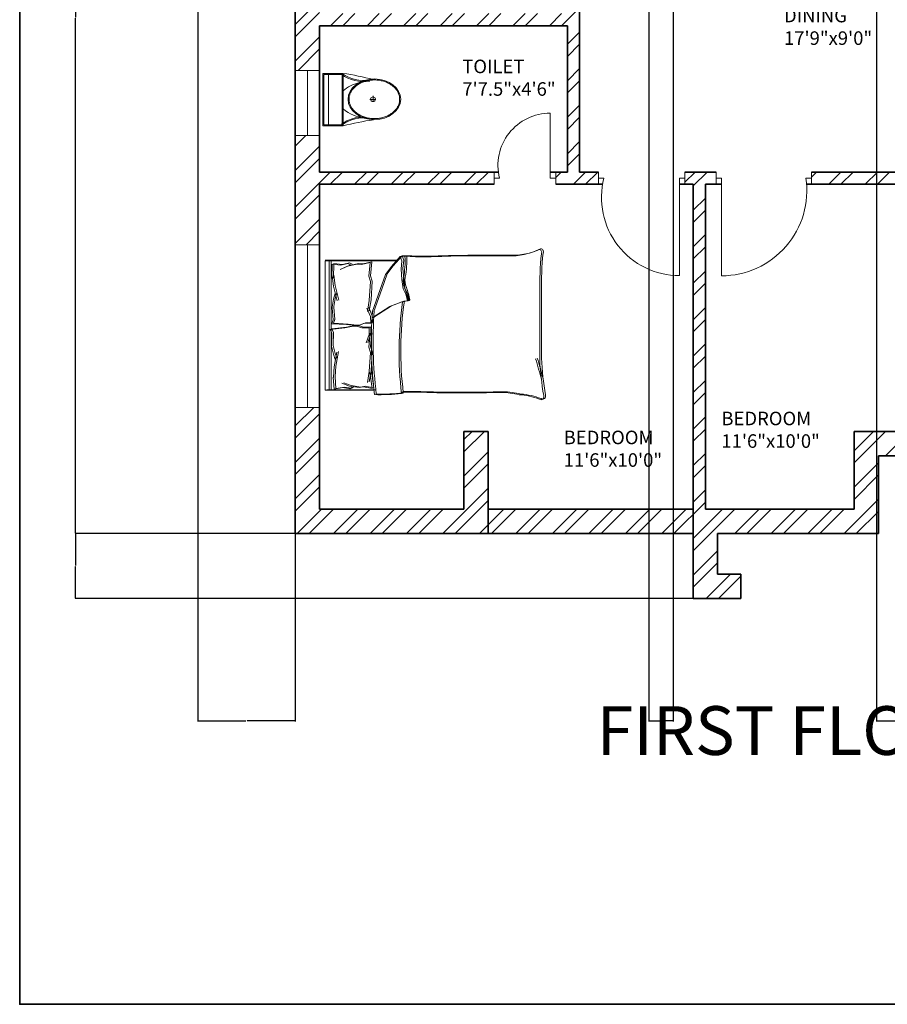
# Model space of a CAD drawing. Units: inches. Extents: x 1513 to 2170, y 1240 to 2288.
# Tile 1 of 10: x 1513 to 1834, y 1240 to 1603. Entities that reach past the tile are written whole.
import ezdxf

# ---------------------------------------------------------------- set-up
doc = ezdxf.new("R2010")
doc.units = ezdxf.units.IN
for name, color, linetype, lineweight in [('A-ANNO-DIMS', 2, 'Continuous', 18), ('A-ANNO-TTLB', 7, 'Continuous', 35), ('A-AREA-IDEN', 7, 'Continuous', 18), ('A-DOOR', 3, 'Continuous', 18), ('A-FLOR-FIXT', 9, 'Continuous', 18), ('A-FURN', 8, 'Continuous', 18), ('A-GLAZ', 4, 'Continuous', 18), ('A-WALL', 7, 'Continuous', 35), ('A-WALL-PATT', 252, 'Continuous', 13)]:
    doc.layers.add(name, color=color, linetype=linetype, lineweight=lineweight)
doc.styles.get("Standard").update_dxf_attribs({"font": 'arial.ttf'})
doc.dimstyles.get("Standard").update_dxf_attribs({"dimtxt": 0.18, "dimasz": 0.18, "dimexe": 0.18, "dimexo": 0.0625, "dimgap": 0.09, "dimtad": 0, "dimtih": 1, "dimtoh": 1, "dimdec": 4, "dimzin": 0, "dimdsep": 46, "dimtxsty": 'Standard', "dimcen": 0.09, "dimadec": 0, "dimazin": 0, "dimtfac": 1, "dimtdec": 4, "dimtofl": 0, "dimtmove": 0, "dimatfit": 3, "dimfxl": 1, "dimtolj": 1, "dimtzin": 0, "dimarcsym": 0})

# ---------------------------------------------------------------- blocks, each defined once
blk = doc.blocks.new('A$C31115884')
for p, q in [((283.1, 497.7), (223.4, 497.7)), ((257.5, 466.4), (257.5, 523.2)), ((0, 200), (0, 0)), ((520, 200), (0, 200)), ((520, 0), (520, 200)), ((10, 190), (10, 10)), ((510, 190), (10, 190)), ((510, 10), (510, 190)), ((510, 54.5), (0, 54.5)), ((10, 10), (510, 10)), ((0, 0), (520, 0))]:
    blk.add_line(p, q)
blk.add_circle((255.6, 496.4), 23.6)
for centre, radius, start, end in [((2777.7, -204.6), 2807, 165.4549, 171.71327), ((3237, 905), 2807, 188.28673, 194.5451), ((-294.5, 403.3), 364.7, 324.20913, 9.34987), ((-294.5, 403.3), 374.7, 324.20913, 9.34987), ((139.5, 406.2), 293.5, 315.84364, 2.65635), ((805.8, 403.3), 374.7, 179.20365, 215.79087), ((805.8, 403.3), 364.7, 170.65013, 215.79087), ((383.6, 406.2), 293.5, 190.27735, 224.15636)]:
    blk.add_arc(centre, radius, start, end)
blk.add_ellipse((256.2, 509.9), major_axis=(0, -260.7), ratio=0.772727)
blk.add_open_spline([(256.2, 259.2), (263.1, 259.2), (270, 259.7), (287.8, 262.3), (298.7, 265.1), (319.9, 273.1), (330.2, 278.4), (350.1, 291.1), (359.7, 298.7), (377.7, 315.9), (386.2, 325.5), (401.7, 346.6), (408.8, 358.1), (421.3, 382.5), (426.8, 395.5), (435.9, 422.4), (439.5, 436.4), (444.8, 465.1), (446.5, 479.7), (447.9, 509.2), (447.6, 524), (445, 553.3), (442.7, 567.8), (436.3, 596), (432.1, 609.7), (421.9, 636), (416, 648.6), (402.5, 672.1), (395, 683), (378.6, 703), (369.8, 712.1), (351.1, 728), (341.3, 734.8), (320.9, 746.2), (310.4, 750.7), (288.9, 757.3), (278, 759.4), (256, 761), (245, 760.6), (223.1, 757.2), (212.3, 754.3), (191.1, 746.1), (180.8, 740.7), (160.9, 727.8), (151.4, 720.1), (133.5, 702.7), (125.1, 693), (109.6, 671.7), (102.6, 660.2), (90.2, 635.7), (84.9, 622.7), (76, 595.6), (72.4, 581.6), (67.2, 552.9), (65.6, 538.2), (64.4, 508.8), (64.8, 494), (67.5, 464.7), (69.9, 450.2), (76.6, 422), (80.8, 408.3), (91.1, 382.2), (97.2, 369.7), (110.8, 346.3), (118.4, 335.4), (134.8, 315.6), (143.7, 306.7), (162.4, 290.9), (172.3, 284.2), (192.8, 273), (203.3, 268.6), (224.8, 262.2), (235.8, 260.2), (249.9, 259.3), (253, 259.2), (256.2, 259.2)], degree=3, knots=[0, 0, 0, 0, 0.110105, 0.110105, 0.285049, 0.285049, 0.459994, 0.459994, 0.634938, 0.634938, 0.809882, 0.809882, 0.984827, 0.984827, 1.159771, 1.159771, 1.334715, 1.334715, 1.50966, 1.50966, 1.684604, 1.684604, 1.859549, 1.859549, 2.034493, 2.034493, 2.209437, 2.209437, 2.384382, 2.384382, 2.559326, 2.559326, 2.73427, 2.73427, 2.909215, 2.909215, 3.084159, 3.084159, 3.259103, 3.259103, 3.434048, 3.434048, 3.608992, 3.608992, 3.783936, 3.783936, 3.958881, 3.958881, 4.133825, 4.133825, 4.30877, 4.30877, 4.483714, 4.483714, 4.658658, 4.658658, 4.833603, 4.833603, 5.008547, 5.008547, 5.183491, 5.183491, 5.358436, 5.358436, 5.53338, 5.53338, 5.708324, 5.708324, 5.883269, 5.883269, 6.058213, 6.058213, 6.233158, 6.233158, 6.283185, 6.283185, 6.283185, 6.283185])
blk = doc.blocks.new('BED-DOUBLE')
for p, q in [((0, 51.27), (26.61, 51.27)), ((0, 51.27), (26.61, 51.27)), ((0.64, 51.49), (27.25, 51.49)), ((0.64, 51.49), (27.25, 51.49)), ((1.53, 3.48), (1.53, 51.27)), ((1.53, 3.48), (1.53, 51.27)), ((2.17, 3.7), (2.17, 51.49)), ((2.17, 3.7), (2.17, 51.49)), ((17.21, 50.93), (14.07, 50.15)), ((17.21, 50.93), (14.07, 50.15)), ((16.8, 45.8), (17.21, 50.93)), ((16.8, 45.8), (17.21, 50.93)), ((27.74, 52.87), (24.49, 49.16)), ((27.74, 52.87), (24.49, 49.16)), ((28.38, 53.1), (25.13, 49.39)), ((28.38, 53.1), (25.13, 49.39)), ((29.49, 52.95), (27.74, 52.87, 3.87)), ((29.49, 52.95), (27.74, 52.87, 3.87)), ((28.36, 51.33), (27.74, 52.87)), ((28.36, 51.33), (27.74, 52.87)), ((28.05, 48.23), (28.36, 51.33)), ((28.05, 48.23), (28.36, 51.33)), ((30.13, 53.18), (28.38, 53.1, 3.87)), ((30.13, 53.18), (28.38, 53.1, 3.87)), ((29, 51.56), (28.38, 53.1)), ((29, 51.56), (28.38, 53.1)), ((28.69, 48.46), (29, 51.56)), ((28.69, 48.46), (29, 51.56)), ((2.55, 50.11), (2.46, 44.71)), ((2.55, 50.11), (2.46, 44.71)), ((2.55, 50.11), (5.76, 49.73)), ((2.55, 50.11), (5.76, 49.73)), ((3.19, 50.34), (3.1, 44.94)), ((3.19, 50.34), (3.1, 44.94)), ((3.19, 50.34), (6.4, 49.96)), ((3.19, 50.34), (6.4, 49.96)), ((8.25, 49.31), (5.57, 48.13)), ((8.25, 49.31), (5.57, 48.13)), ((5.76, 49.73), (8.33, 50.33)), ((5.76, 49.73), (8.33, 50.33)), ((8.89, 49.54), (6.21, 48.36)), ((8.89, 49.54), (6.21, 48.36)), ((6.4, 49.96), (8.97, 50.56)), ((6.4, 49.96), (8.97, 50.56)), ((11.83, 50.11), (8.25, 49.31)), ((11.83, 50.11), (8.25, 49.31)), ((8.33, 50.33), (9.38, 49.82)), ((8.33, 50.33), (9.38, 49.82)), ((12.46, 50.34), (8.89, 49.54)), ((12.46, 50.34), (8.89, 49.54)), ((8.97, 50.56), (10.02, 50.04)), ((8.97, 50.56), (10.02, 50.04)), ((13.43, 49.92), (11.83, 50.11)), ((13.43, 49.92), (11.83, 50.11)), ((14.07, 50.15), (12.46, 50.34)), ((14.07, 50.15), (12.46, 50.34)), ((16.57, 50.7), (13.43, 49.92)), ((16.57, 50.7), (13.43, 49.92)), ((16.17, 45.57), (16.57, 50.7)), ((16.17, 45.57), (16.57, 50.7)), ((24.49, 49.16), (22.33, 46.22)), ((24.49, 49.16), (22.33, 46.22)), ((25.13, 49.39), (22.96, 46.45)), ((25.13, 49.39), (22.96, 46.45)), ((28.36, 44.36), (28.05, 48.23)), ((28.36, 44.36), (28.05, 48.23)), ((29, 44.59), (28.69, 48.46)), ((29, 44.59), (28.69, 48.46)), ((2.46, 44.71), (2.54, 45.71)), ((2.46, 44.71), (2.54, 45.71)), ((2.54, 45.71), (3.07, 41.92)), ((2.54, 45.71), (3.07, 41.92)), ((3.1, 44.94), (3.18, 45.94)), ((3.1, 44.94), (3.18, 45.94)), ((3.18, 45.94), (3.71, 42.14)), ((3.18, 45.94), (3.71, 42.14)), ((16.72, 43.61), (16.17, 45.57)), ((16.72, 43.61), (16.17, 45.57)), ((17.36, 43.84), (16.8, 45.8)), ((17.36, 43.84), (16.8, 45.8)), ((16.93, 36.83), (17.36, 43.84)), ((16.93, 36.83), (17.36, 43.84)), ((22.33, 46.22), (20.31, 40.65)), ((22.33, 46.22), (20.31, 40.65)), ((22.96, 46.45), (20.95, 40.87)), ((22.96, 46.45), (20.95, 40.87)), ((28.83, 40.96), (28.36, 44.36)), ((28.83, 40.95), (28.36, 44.36)), ((29.46, 41.18), (29, 44.59)), ((29.46, 41.18), (29, 44.59)), ((3.07, 41.92), (4.42, 36.5)), ((3.07, 41.92), (4.42, 36.5)), ((3.71, 42.14), (5.06, 36.72)), ((3.71, 42.14), (5.06, 36.72)), ((16.29, 36.6), (16.72, 43.61)), ((16.29, 36.6), (16.72, 43.61)), ((20.31, 40.65), (17.38, 32.31)), ((20.31, 40.65), (17.38, 32.31)), ((20.95, 40.87), (18.02, 32.54)), ((20.95, 40.87), (18.02, 32.54)), ((29.75, 38.94), (28.83, 40.96)), ((29.75, 38.94), (28.83, 40.95)), ((30.39, 39.17), (29.46, 41.18)), ((30.39, 39.17), (29.46, 41.18)), ((3.07, 37.14), (2.53, 34.21)), ((3.07, 37.14), (2.53, 34.21)), ((3.67, 39.2), (3.07, 37.14)), ((3.67, 39.2), (3.07, 37.14)), ((3.71, 37.36), (3.17, 34.43)), ((3.71, 37.36), (3.17, 34.43)), ((4.31, 39.43), (3.71, 37.36)), ((4.31, 39.43), (3.71, 37.36)), ((15.62, 32.57), (16.29, 36.6)), ((15.62, 32.57), (16.29, 36.6)), ((16.26, 32.79), (16.93, 36.83)), ((16.26, 32.79), (16.93, 36.83)), ((24.51, 34.68), (29, 36.38)), ((24.51, 34.68), (29, 36.38)), ((28.36, 36.15), (30.37, 36.46)), ((28.36, 36.15), (30.37, 36.46)), ((29, 36.38), (31.01, 36.69)), ((29, 36.38), (31.01, 36.69)), ((30.37, 36.46), (29.75, 38.94)), ((30.37, 36.46), (29.75, 38.94)), ((31.01, 36.69), (30.39, 39.17)), ((31.01, 36.69), (30.39, 39.17)), ((79.24, 15.06), (79.24, 39.68)), ((79.24, 15.06), (79.24, 39.68)), ((79.88, 15.29), (79.88, 39.91)), ((79.88, 15.29), (79.88, 39.91)), ((2.53, 34.21), (2.55, 33.88)), ((2.53, 34.21), (2.55, 33.88)), ((2.55, 33.88), (2.98, 29.46)), ((2.55, 33.88), (2.98, 29.46)), ((3.17, 34.43), (3.19, 34.11)), ((3.17, 34.43), (3.19, 34.11)), ((3.19, 34.11), (3.61, 29.69)), ((3.19, 34.11), (3.61, 29.68)), ((16.74, 30.75), (15.45, 33.82)), ((16.74, 30.75), (15.45, 33.82)), ((17.38, 30.98), (16.09, 34.05)), ((17.38, 30.98), (16.09, 34.05)), ((17.38, 30.26), (23.87, 34.45)), ((17.38, 30.26), (23.87, 34.45)), ((18.02, 30.49), (24.51, 34.68)), ((18.02, 30.49), (24.51, 34.68)), ((23.87, 34.45), (28.36, 36.15)), ((23.87, 34.45), (28.36, 36.15)), ((2.98, 29.46), (2.49, 27.98)), ((2.98, 29.46), (2.49, 27.98)), ((3.61, 29.69), (3.13, 28.21)), ((3.61, 29.68), (3.13, 28.21)), ((16.89, 28.3), (16.74, 30.75)), ((16.89, 28.3), (16.74, 30.75)), ((17.53, 28.53), (17.38, 30.98)), ((17.53, 28.53), (17.38, 30.98)), ((1.87, 25.98), (7.22, 26.56)), ((1.87, 25.98), (7.22, 26.56)), ((2.44, 24.54), (1.87, 25.98)), ((2.44, 24.54), (1.87, 25.98)), ((2.49, 27.98), (7.86, 27.73)), ((2.49, 27.98), (7.86, 27.73)), ((2.51, 26.21), (7.86, 26.79)), ((2.51, 26.21), (7.86, 26.79)), ((3.08, 24.77), (2.51, 26.21)), ((3.08, 24.77), (2.51, 26.21)), ((3.13, 28.21), (8.5, 27.96)), ((3.13, 28.21), (8.5, 27.96)), ((7.22, 26.56), (10.4, 27.14)), ((7.22, 26.56), (10.4, 27.14)), ((7.86, 27.73), (11.07, 27.36)), ((7.86, 27.73), (11.07, 27.36)), ((7.86, 26.79), (11.04, 27.37)), ((7.86, 26.79), (11.04, 27.37)), ((8.5, 27.96), (11.71, 27.58)), ((8.5, 27.96), (11.71, 27.58)), ((10.4, 27.14), (11.7, 27.14)), ((10.4, 27.14), (11.7, 27.14)), ((11.04, 27.37), (12.34, 27.37)), ((11.04, 27.37), (12.34, 27.37)), ((11.07, 27.36), (12.37, 27.44)), ((11.07, 27.36), (12.37, 27.44)), ((11.7, 27.14), (13.58, 26.56)), ((11.7, 27.14), (13.58, 26.56)), ((11.71, 27.58), (13.01, 27.67)), ((11.71, 27.58), (13.01, 27.67)), ((12.34, 27.37), (14.22, 26.79)), ((12.34, 27.37), (14.22, 26.79)), ((12.37, 27.44), (14.21, 28.13)), ((12.37, 27.44), (14.21, 28.13)), ((13.01, 27.67), (14.85, 28.36)), ((13.01, 27.67), (14.85, 28.36)), ((13.58, 26.56), (16.26, 26.56)), ((13.58, 26.56), (16.26, 26.56)), ((14.21, 28.13), (16.89, 28.3)), ((14.21, 28.13), (16.89, 28.3)), ((14.22, 26.79), (16.9, 26.79)), ((14.22, 26.79), (16.9, 26.79)), ((14.85, 28.36), (17.53, 28.53)), ((14.85, 28.36), (17.53, 28.53)), ((16.26, 26.56), (16.26, 24.1)), ((16.26, 26.56), (16.26, 24.1)), ((16.9, 26.79), (16.9, 24.33)), ((16.9, 26.79), (16.9, 24.33)), ((2.3, 20.09), (2.44, 24.54)), ((2.3, 20.09), (2.44, 24.54)), ((2.94, 20.32), (3.08, 24.77)), ((2.94, 20.32), (3.08, 24.77)), ((16.26, 24.1), (15.17, 20.96)), ((16.26, 24.1), (15.17, 20.96)), ((16.9, 24.33), (15.81, 21.19)), ((16.9, 24.33), (15.81, 21.19)), ((16.17, 19.39), (16.57, 24.52)), ((16.17, 19.38), (16.57, 24.52)), ((16.8, 19.61), (17.21, 24.75)), ((16.8, 19.61), (17.21, 24.74)), ((2.3, 19.77), (2.3, 20.09)), ((2.3, 19.77), (2.3, 20.09)), ((3.02, 16.88), (2.3, 19.77)), ((3.02, 16.88), (2.3, 19.77)), ((2.94, 20), (2.94, 20.32)), ((2.94, 20), (2.94, 20.32)), ((3.66, 17.11), (2.94, 20)), ((3.66, 17.11), (2.94, 20)), ((16.72, 17.42), (16.17, 19.39)), ((16.72, 17.42), (16.17, 19.38)), ((17.36, 17.65), (16.8, 19.61)), ((17.36, 17.65), (16.8, 19.61)), ((3.75, 14.86), (3.02, 16.88)), ((3.75, 14.86), (3.02, 16.88)), ((3.31, 12.11), (4.32, 17.6)), ((3.31, 12.11), (4.32, 17.6)), ((4.39, 15.08), (3.66, 17.11)), ((4.39, 15.08), (3.66, 17.11)), ((3.95, 12.34), (4.96, 17.83)), ((3.95, 12.34), (4.96, 17.83)), ((16.29, 10.41), (16.72, 17.42)), ((16.29, 10.41), (16.72, 17.42)), ((16.93, 10.64), (17.36, 17.65)), ((16.93, 10.64), (17.36, 17.65)), ((3.02, 8.29), (3.31, 12.11)), ((3.02, 8.29), (3.31, 12.11)), ((3.66, 8.51), (3.95, 12.34)), ((3.66, 8.51), (3.95, 12.34)), ((3.01, 8.18), (3.02, 8.29)), ((3.01, 8.18), (3.02, 8.29)), ((3.33, 3.9), (3.01, 8.18)), ((3.33, 3.9), (3.01, 8.18)), ((3.64, 8.41), (3.66, 8.51)), ((3.64, 8.41), (3.66, 8.51)), ((3.97, 4.13), (3.64, 8.41)), ((3.97, 4.13), (3.64, 8.41)), ((15.62, 6.38), (16.29, 10.41)), ((15.62, 6.38), (16.29, 10.41)), ((16.26, 6.61), (16.93, 10.64)), ((16.26, 6.61), (16.93, 10.64)), ((16.29, 10.41), (16.61, 9.28)), ((16.29, 10.41), (16.61, 9.28)), ((16.61, 9.28), (17.34, 4.18)), ((16.61, 9.28), (17.34, 4.18)), ((16.93, 10.64), (17.25, 9.51)), ((16.93, 10.64), (17.25, 9.51)), ((17.25, 9.51), (17.98, 4.41)), ((17.25, 9.51), (17.98, 4.41)), ((18.75, 3.7), (0.64, 3.7)), ((18.75, 3.7), (0.64, 3.7)), ((3.31, 3.9), (6.49, 4.47)), ((3.31, 3.9), (6.49, 4.47)), ((3.95, 4.12), (7.13, 4.7)), ((3.95, 4.12), (7.13, 4.7)), ((8.95, 5.05), (6.2, 6.06)), ((8.95, 5.05), (6.2, 6.06)), ((6.49, 4.47), (9.1, 4.04)), ((6.49, 4.47), (9.1, 4.04)), ((9.59, 5.28), (6.84, 6.29)), ((9.59, 5.28), (6.84, 6.29)), ((7.13, 4.7), (9.74, 4.27)), ((7.13, 4.7), (9.74, 4.27)), ((12.57, 4.47), (8.95, 5.05)), ((12.57, 4.47), (8.95, 5.05)), ((9.1, 4.04), (10.11, 4.62)), ((9.1, 4.04), (10.11, 4.62)), ((13.21, 4.7), (9.59, 5.28)), ((13.21, 4.7), (9.59, 5.28)), ((9.74, 4.27), (10.75, 4.85)), ((9.74, 4.27), (10.75, 4.85)), ((14.16, 4.76), (12.57, 4.47)), ((14.16, 4.76), (12.57, 4.47)), ((14.8, 4.99), (13.21, 4.7)), ((14.8, 4.99), (13.21, 4.7)), ((17.34, 4.18), (14.16, 4.76)), ((17.34, 4.18), (14.16, 4.76)), ((17.98, 4.41), (14.8, 4.99)), ((17.98, 4.41), (14.8, 4.99)), ((18.11, 3.48), (0, 3.48)), ((18.11, 3.48), (0, 3.48))]:
    blk.add_line(p, q)
for centre, radius, start, end in [((68.66, 76.16), 23.07, 267.4714, 296.4681), ((68.66, 76.16), 23.07, 267.4714, 296.4681), ((69.3, 76.39), 23.07, 267.4714, 296.4681), ((69.3, 76.39), 23.07, 267.4714, 296.4681), ((78.87, 54.41), 1.1, 332.6588, 86.02), ((78.87, 54.41), 1.1, 332.6588, 86.02), ((79.51, 54.64), 1.1, 332.6588, 86.02), ((79.51, 54.64), 1.1, 332.6588, 86.02), ((-6.66, 51.33), 36.18, 349.8763, 2.5657), ((-6.66, 51.33), 36.18, 349.8763, 2.5657), ((36.31, 182.27), 129.5, 266.9791, 273.8365), ((36.31, 182.27), 129.5, 266.9791, 273.8365), ((-6.02, 51.56), 36.18, 349.8763, 2.5657), ((-6.02, 51.56), 36.18, 349.8763, 2.5657), ((36.95, 182.5), 129.5, 266.9791, 273.8365), ((36.95, 182.5), 129.5, 266.9791, 273.8365), ((67.82, -4508.74), 4561.86, 90.00217, 90.28689), ((67.82, -4508.74), 4561.86, 90.00217, 90.28689), ((68.46, -4508.51), 4561.86, 90.00217, 90.28689), ((68.46, -4508.51), 4561.86, 90.00217, 90.28689), ((212.27, 41.15), 133.04, 174.4998, 180.6351), ((212.27, 41.15), 133.04, 174.4998, 180.6351), ((212.91, 41.38), 133.04, 174.4998, 180.6351), ((212.91, 41.38), 133.04, 174.4998, 180.6351), ((35.06, 43.74), 6.22, 168.6608, 203.7384), ((35.06, 43.74), 6.22, 168.6608, 203.7384), ((35.7, 43.97), 6.22, 168.6608, 203.7384), ((35.7, 43.97), 6.22, 168.6608, 203.7384), ((1.48, 31.15), 29.65, 10.6617, 19.8806), ((1.48, 31.15), 29.65, 10.6617, 19.8806), ((2.12, 31.38), 29.65, 10.6617, 19.8806), ((2.12, 31.38), 29.65, 10.6617, 19.8806), ((156.95, 17.99), 129.02, 171.7845, 186.9006), ((156.95, 17.98), 129.02, 171.7845, 186.9006), ((30.44, 36.64), 0.185, 250.2464, 1.1377), ((30.44, 36.64), 0.185, 250.2464, 1.1377), ((31.08, 36.87), 0.185, 250.2464, 1.1377), ((31.08, 36.87), 0.185, 250.2464, 1.1377), ((182.69, 21.59), 164.97, 176.0865, 186.7821), ((182.69, 21.59), 164.97, 176.0865, 186.7821), ((156.31, 17.76), 129.02, 171.7845, 186.9006), ((156.31, 17.76), 129.02, 171.7845, 186.9006), ((182.05, 21.36), 164.97, 176.0865, 186.7821), ((182.05, 21.36), 164.97, 176.0865, 186.7821), ((-23.72, -17.22), 106.46, 13.3832, 17.7053), ((-23.72, -17.22), 106.46, 13.3832, 17.7053), ((-23.08, -16.99), 106.46, 13.3832, 17.7053), ((-23.08, -16.99), 106.46, 13.3832, 17.7053), ((200.83, 21.43), 121.76, 182.9958, 189.4091), ((200.83, 21.43), 121.76, 182.9958, 189.4091), ((201.47, 21.66), 121.76, 182.9958, 189.4091), ((201.47, 21.66), 121.76, 182.9958, 189.4091), ((20.09, 85.16), 83.31, 268.7218, 275.604), ((20.09, 85.16), 83.31, 268.7218, 275.604), ((20.73, 85.39), 83.31, 268.7218, 275.604), ((20.73, 85.39), 83.31, 268.7218, 275.604), ((31.17, -167.31), 170.11, 88.4762, 91.0082), ((31.17, -167.31), 170.11, 88.4762, 91.0082), ((31.81, -167.08), 170.11, 88.4762, 91.0082), ((31.81, -167.08), 170.11, 88.4762, 91.0082), ((50.61, 484.82), 482.31, 268.2277, 271.7185), ((50.61, 484.82), 482.31, 268.2277, 271.7185), ((51.25, 485.05), 482.31, 268.2277, 271.7185), ((51.25, 485.05), 482.31, 268.2277, 271.7185), ((64.51, -26.9), 29.63, 76.0648, 88.9113), ((64.51, -26.9), 29.63, 76.0648, 88.9113), ((65.15, -26.67), 29.63, 76.0648, 88.9113), ((65.15, -26.67), 29.63, 76.0648, 88.9113), ((70.27, -21.66), 23.56, 67.9751, 86.652), ((70.27, -21.66), 23.56, 67.9751, 86.652), ((70.91, -21.43), 23.56, 67.9751, 86.652), ((70.91, -21.43), 23.56, 67.9751, 86.652), ((79.71, 1.09), 1.09, 236.1736, 23.4781), ((79.71, 1.09), 1.09, 236.1736, 23.4781), ((80.35, 1.32), 1.09, 236.1736, 23.4781), ((80.35, 1.32), 1.09, 236.1736, 23.4781)]:
    blk.add_arc(centre, radius, start, end)
blk = doc.blocks.new('WIN-24-ALT')
for p, q in [((4.5, 24), (0, 24)), ((0, 24), (9, 24)), ((4.5, 0), (4.5, 24)), ((9, 0), (0, 0)), ((0, 0), (4.5, 0))]:
    blk.add_line(p, q)
blk = doc.blocks.new('*D27')
at = {"layer": 'A-ANNO-DIMS', "color": 0, "lineweight": -2, "transparency": 16777216}
for p, q in [((1578.87, 1956.42), (1578.87, 1344.15)), ((1614.87, 1956.42), (1614.87, 1344.15)), ((1579.05, 1344.33), (1596.65, 1344.33)), ((1614.69, 1344.33), (1597.08, 1344.33))]:
    blk.add_line(p, q, dxfattribs=at)
at = {"layer": 'A-ANNO-DIMS', "color": 0, "transparency": 16777216}
for points in [[(1579.05, 1344.36), (1579.05, 1344.3), (1578.87, 1344.33)], [(1614.69, 1344.36), (1614.69, 1344.3), (1614.87, 1344.33)]]:
    blk.add_solid(points, dxfattribs=at)
at = {"layer": 'Defpoints', "color": 0, "transparency": 16777216}
for p in [(1578.87, 1956.48), (1614.87, 1956.48), (1614.87, 1344.33)]:
    blk.add_point(p, dxfattribs=at)
at = {"layer": 'A-ANNO-DIMS', "color": 0, "transparency": 16777216, "insert": (1596.87, 1344.33), "char_height": 0.18, "attachment_point": 5}
blk.add_mtext('\\A1;36', dxfattribs=at)
blk = doc.blocks.new('*D29')
at = {"layer": 'A-ANNO-DIMS', "color": 0, "lineweight": -2, "transparency": 16777216}
for p, q in [((1578.8, 1794.48), (1533.54, 1794.48)), ((1533.72, 1794.3), (1533.72, 1604.16)), ((1533.72, 1413.66), (1533.72, 1603.8)), ((1614.8, 1413.48), (1533.54, 1413.48))]:
    blk.add_line(p, q, dxfattribs=at)
at = {"layer": 'A-ANNO-DIMS', "color": 0, "transparency": 16777216}
for points in [[(1533.69, 1794.3), (1533.75, 1794.3), (1533.72, 1794.48)], [(1533.69, 1413.66), (1533.75, 1413.66), (1533.72, 1413.48)]]:
    blk.add_solid(points, dxfattribs=at)
at = {"layer": 'Defpoints', "color": 0, "transparency": 16777216}
for p in [(1533.72, 1794.48), (1578.87, 1794.48), (1614.87, 1413.48)]:
    blk.add_point(p, dxfattribs=at)
at = {"layer": 'A-ANNO-DIMS', "color": 0, "transparency": 16777216, "insert": (1533.72, 1603.98), "char_height": 0.18, "attachment_point": 5}
blk.add_mtext('\\A1;381', dxfattribs=at)
blk = doc.blocks.new('*D31')
at = {"layer": 'A-ANNO-DIMS', "color": 0, "lineweight": -2, "transparency": 16777216}
for p, q in [((1614.8, 1413.48), (1533.54, 1413.48)), ((1533.72, 1413.3), (1533.72, 1401.66)), ((1533.72, 1389.66), (1533.72, 1401.3)), ((1761.8, 1389.48), (1533.54, 1389.48))]:
    blk.add_line(p, q, dxfattribs=at)
at = {"layer": 'A-ANNO-DIMS', "color": 0, "transparency": 16777216}
for points in [[(1533.69, 1413.3), (1533.75, 1413.3), (1533.72, 1413.48)], [(1533.69, 1389.66), (1533.75, 1389.66), (1533.72, 1389.48)]]:
    blk.add_solid(points, dxfattribs=at)
at = {"layer": 'Defpoints', "color": 0, "transparency": 16777216}
for p in [(1533.72, 1413.48), (1614.87, 1413.48), (1761.87, 1389.48)]:
    blk.add_point(p, dxfattribs=at)
at = {"layer": 'A-ANNO-DIMS', "color": 0, "transparency": 16777216, "insert": (1533.72, 1401.48), "char_height": 0.18, "attachment_point": 5}
blk.add_mtext('\\A1;24', dxfattribs=at)
blk = doc.blocks.new('*D34')
at = {"layer": 'A-ANNO-DIMS', "color": 0, "lineweight": -2, "transparency": 16777216}
for p, q in [((1745.46, 1803.42), (1745.46, 1344.15)), ((1754.46, 1803.42), (1754.46, 1344.15)), ((1745.64, 1344.33), (1749.81, 1344.33)), ((1754.28, 1344.33), (1750.11, 1344.33))]:
    blk.add_line(p, q, dxfattribs=at)
at = {"layer": 'A-ANNO-DIMS', "color": 0, "transparency": 16777216}
for points in [[(1745.64, 1344.36), (1745.64, 1344.3), (1745.46, 1344.33)], [(1754.28, 1344.36), (1754.28, 1344.3), (1754.46, 1344.33)]]:
    blk.add_solid(points, dxfattribs=at)
at = {"layer": 'Defpoints', "color": 0, "transparency": 16777216}
for p in [(1745.46, 1803.48), (1754.46, 1803.48), (1754.46, 1344.33)]:
    blk.add_point(p, dxfattribs=at)
at = {"layer": 'A-ANNO-DIMS', "color": 0, "transparency": 16777216, "insert": (1749.96, 1344.33), "char_height": 0.18, "attachment_point": 5}
blk.add_mtext('\\A1;9', dxfattribs=at)
blk = doc.blocks.new('*D36')
at = {"layer": 'A-ANNO-DIMS', "color": 0, "lineweight": -2, "transparency": 16777216}
for p, q in [((1829.49, 1887.42), (1829.49, 1344.15)), ((1864.51, 1887.42), (1864.51, 1344.15)), ((1829.67, 1344.33), (1846.61, 1344.33)), ((1864.33, 1344.33), (1847.39, 1344.33))]:
    blk.add_line(p, q, dxfattribs=at)
at = {"layer": 'A-ANNO-DIMS', "color": 0, "transparency": 16777216}
for points in [[(1829.67, 1344.36), (1829.67, 1344.3), (1829.49, 1344.33)], [(1864.33, 1344.36), (1864.33, 1344.3), (1864.51, 1344.33)]]:
    blk.add_solid(points, dxfattribs=at)
at = {"layer": 'Defpoints', "color": 0, "transparency": 16777216}
for p in [(1829.49, 1887.48), (1864.51, 1887.48), (1864.51, 1344.33)]:
    blk.add_point(p, dxfattribs=at)
at = {"layer": 'A-ANNO-DIMS', "color": 0, "transparency": 16777216, "insert": (1847, 1344.33), "char_height": 0.18, "attachment_point": 5}
blk.add_mtext('\\A1;35.02', dxfattribs=at)

msp = doc.modelspace()

# ---------------------------------------------------------------- hatches: boundary and pattern name
at = {"layer": 'A-WALL-PATT'}
h = msp.add_hatch(dxfattribs=at)
h.set_pattern_fill('ANSI32', color=256)
h.paths.add_polyline_path([(2041.852, 1719.48), (2014.852, 1719.48), (2014.852, 1734.444), (2005.852, 1734.444), (2005.852, 1710.48), (2032.852, 1710.48), (2032.852, 1663.98), (1976.619, 1663.98), (1976.619, 1659.48), (2005.852, 1659.48), (2005.852, 1626.27), (2014.852, 1626.27), (2014.852, 1659.48), (2041.852, 1659.48)])
h.paths.add_polyline_path([(1954.521, 1663.98), (1875.357, 1663.98), (1875.357, 1659.48), (1945.852, 1659.48), (1945.852, 1546.98), (1950.352, 1546.98), (2005.852, 1546.98), (2005.852, 1422.48), (1985.47, 1422.48), (1985.47, 1413.48), (2014.852, 1413.48), (2014.852, 1602.27), (2005.852, 1602.27), (2005.852, 1551.48), (1950.352, 1551.48), (1950.352, 1659.48), (1954.521, 1659.48)])
h.paths.add_polyline_path([(1949.47, 1422.48), (1937.366, 1422.48), (1937.366, 1413.48), (1949.47, 1413.48)], flags=0)
h.paths.add_polyline_path([(1937.366, 1422.48), (1908.866, 1422.48), (1908.866, 1546.98), (1805.486, 1546.98), (1805.486, 1542.48), (1904.366, 1542.48), (1904.366, 1451.2), (1897.222, 1451.2), (1897.222, 1442.2), (1904.366, 1442.2), (1904.366, 1422.48), (1904.366, 1413.48), (1904.366, 1389.48), (1908.866, 1389.48), (1908.866, 1413.48), (1932.866, 1413.48), (1932.866, 1389.48), (1937.366, 1389.48)])
h.paths.add_polyline_path([(1830.254, 1442.2), (1844.144, 1442.2), (1844.144, 1451.2), (1830.254, 1451.2), (1821.254, 1451.2), (1821.254, 1422.48), (1766.366, 1422.48), (1766.366, 1542.48), (1770.265, 1542.48), (1770.265, 1546.98), (1758.774, 1546.98), (1758.774, 1544.73), (1758.774, 1542.48), (1761.866, 1542.48), (1761.866, 1389.48), (1779.454, 1389.48), (1779.454, 1398.48), (1770.866, 1398.48), (1770.866, 1413.48), (1830.254, 1413.48)])
h.paths.add_polyline_path([(1686.156, 1451.2), (1677.156, 1451.2), (1677.156, 1422.48), (1623.866, 1422.48), (1623.866, 1460.073), (1614.866, 1460.073), (1614.866, 1413.48), (1686.156, 1413.48)])
h.paths.add_polyline_path([(1761.866, 1422.48), (1686.156, 1422.48), (1686.156, 1413.48), (1761.866, 1413.48)])
h.paths.add_polyline_path([(1623.866, 1542.48), (1688.266, 1542.48), (1688.266, 1544.73), (1688.266, 1546.98), (1623.866, 1546.98), (1623.866, 1560.442), (1614.866, 1560.442), (1614.866, 1520.073), (1619.366, 1520.073), (1623.866, 1520.073)])
h.paths.add_polyline_path([(1623.866, 1600.98), (1715.366, 1600.98), (1715.366, 1546.98), (1711.055, 1546.98), (1711.055, 1542.48), (1719.866, 1542.48), (1726.867, 1542.48), (1726.867, 1544.73), (1726.867, 1546.98), (1719.866, 1546.98), (1719.866, 1600.98), (1719.866, 1608.301), (1717.616, 1608.301), (1715.366, 1608.301), (1715.366, 1605.48), (1623.866, 1605.48), (1623.866, 1620.254), (1614.866, 1620.254), (1614.866, 1584.442), (1623.866, 1584.442)])
h.paths.add_polyline_path([(1623.866, 1659.48), (1715.366, 1659.48), (1715.366, 1629.2), (1719.866, 1629.2), (1719.866, 1659.48), (1767.866, 1659.48), (1767.866, 1629.2), (1772.366, 1629.2), (1772.366, 1663.98), (1578.866, 1663.98), (1578.866, 1661.73), (1578.866, 1659.48), (1578.866, 1635.48), (1583.366, 1635.48), (1583.366, 1654.98), (1614.866, 1654.98), (1614.866, 1644.254), (1619.366, 1644.254), (1623.866, 1644.254)])
h.paths.add_polyline_path([(1788.587, 1798.98), (1788.587, 1803.48), (1623.866, 1803.48), (1623.866, 1887.48), (1829.49, 1887.48), (1829.49, 1891.98), (1829.49, 1896.48), (1748.366, 1896.48), (1743.866, 1896.48), (1623.866, 1896.48), (1623.866, 1904.333), (1619.366, 1904.333), (1614.866, 1904.333), (1614.866, 1896.48), (1578.866, 1896.48), (1578.866, 1887.48), (1614.866, 1887.48), (1614.866, 1803.48), (1578.866, 1803.48), (1578.866, 1794.48), (1626.866, 1794.48), (1788.587, 1794.48)])
h.paths.add_polyline_path([(1635.866, 1794.48), (1626.866, 1794.48), (1626.866, 1763.627), (1631.366, 1763.627), (1635.866, 1763.627)])
h.paths.add_polyline_path([(1635.866, 1703.627), (1626.866, 1703.627), (1626.866, 1663.98), (1635.866, 1663.98)])
h.paths.add_polyline_path([(1587.866, 2016.48), (1614.866, 2016.48), (1623.866, 2016.48), (1707.767, 2016.48), (1707.767, 2018.73), (1707.767, 2020.98), (1706.366, 2020.98), (1706.366, 2025.944), (1701.866, 2025.944), (1701.866, 2020.98), (1623.866, 2020.98), (1623.866, 2045.903), (1614.866, 2045.903), (1614.866, 2025.48), (1583.366, 2025.48), (1583.366, 2040.48), (1578.866, 2040.48), (1578.866, 2016.48), (1578.866, 1956.48), (1614.866, 1956.48), (1614.866, 1946.333), (1623.866, 1946.333), (1623.866, 1965.48), (1587.866, 1965.48)])
h.paths.add_polyline_path([(1748.366, 2016.48), (1748.366, 2025.48), (1743.866, 2025.48), (1739.366, 2025.48), (1739.366, 2020.98), (1738.09, 2020.98), (1738.09, 2016.48), (1743.866, 2016.48), (1743.866, 1896.48), (1748.366, 1896.48)])
h.paths.add_polyline_path([(1746.736, 2085.48), (1623.866, 2085.48), (1623.866, 2205.48), (1657.136, 2205.48), (1657.136, 2214.48), (1614.866, 2214.48), (1614.866, 2069.903), (1623.866, 2069.903), (1623.866, 2080.98), (1683.866, 2080.98), (1701.866, 2080.98), (1701.866, 2046.743), (1706.366, 2046.743), (1706.366, 2080.98), (1746.736, 2080.98)])

# ---------------------------------------------------------------- linework, layer by layer
at = {"layer": 'A-ANNO-TTLB'}
msp.add_lwpolyline([(1513.071, 2287.731), (2170.435, 2287.731), (2170.435, 1239.669), (1513.071, 1239.669)], close=True, dxfattribs=at)
at = {"layer": 'A-DOOR'}
for p, q in [((1709.055, 1544.73), (1709.055, 1568.73)), ((1688.266, 1546.98), (1688.266, 1542.48)), ((1711.055, 1546.98), (1711.055, 1542.48)), ((1726.867, 1546.98), (1726.867, 1542.48)), ((1758.774, 1542.48), (1758.774, 1546.98)), ((1758.774, 1546.98), (1758.774, 1544.73)), ((1770.265, 1542.48), (1770.265, 1546.98)), ((1770.265, 1546.98), (1770.265, 1544.663)), ((1805.486, 1546.98), (1805.486, 1542.48)), ((1688.266, 1542.48), (1688.266, 1544.73)), ((1688.266, 1544.73), (1690.266, 1544.73)), ((1711.055, 1544.73), (1709.055, 1544.73)), ((1711.055, 1542.48), (1711.055, 1544.73)), ((1726.867, 1542.48), (1726.867, 1544.73)), ((1726.867, 1544.73), (1728.867, 1544.73)), ((1758.774, 1544.73), (1756.774, 1544.73)), ((1756.774, 1544.73), (1756.774, 1508.73)), ((1770.265, 1544.663), (1772.265, 1544.663)), ((1772.265, 1544.663), (1772.265, 1508.663)), ((1805.486, 1544.73), (1803.486, 1544.73)), ((1805.486, 1542.48), (1805.486, 1544.73))]:
    msp.add_line(p, q, dxfattribs=at)
for centre, radius, start, end in [((1709.055, 1549.375), 19.355, 90, 193.88759), ((1756.774, 1537.546), 28.816, 165.56428, 270), ((1772.265, 1540.209), 31.547, 270, 8.23823)]:
    msp.add_arc(centre, radius, start, end, dxfattribs=at)
at = {"layer": 'A-FURN'}
for p, q in [((1625.893, 1514.398), (1626.532, 1514.398)), ((1625.893, 1514.169), (1625.893, 1466.379))]:
    msp.add_line(p, q, dxfattribs=at)
at = {"layer": 'A-GLAZ'}
for p, q in [((1623.866, 1520.073), (1614.866, 1520.073)), ((1614.866, 1520.073), (1619.366, 1520.073)), ((1619.366, 1520.073), (1619.366, 1460.073)), ((1623.866, 1460.073), (1614.866, 1460.073)), ((1619.366, 1460.073), (1623.866, 1460.073))]:
    msp.add_line(p, q, dxfattribs=at)
at = {"layer": 'A-WALL'}
for p, q in [((1614.866, 1654.98), (1614.866, 1413.48)), ((1719.866, 1600.98), (1719.866, 1609.123)), ((1623.866, 1600.98), (1715.366, 1600.98)), ((1623.866, 1600.98), (1623.866, 1546.98)), ((1623.866, 1600.98), (1623.866, 1546.98)), ((1715.366, 1546.98), (1715.366, 1600.98)), ((1719.866, 1546.98), (1719.866, 1600.98)), ((1623.866, 1546.98), (1689.849, 1546.98)), ((1709.055, 1546.98), (1715.366, 1546.98)), ((1719.866, 1546.98), (1726.867, 1546.98)), ((1758.774, 1546.98), (1770.265, 1546.98)), ((1761.866, 1546.98), (1766.366, 1546.98)), ((1805.486, 1546.98), (1908.866, 1546.98)), ((1623.866, 1542.48), (1688.266, 1542.48)), ((1623.866, 1542.48), (1623.866, 1422.48)), ((1711.055, 1542.48), (1719.866, 1542.48)), ((1719.866, 1542.48), (1715.366, 1542.48)), ((1728.383, 1542.48), (1719.866, 1542.48)), ((1761.866, 1542.48), (1756.774, 1542.48)), ((1761.866, 1389.48), (1761.866, 1542.48)), ((1766.366, 1542.48), (1766.366, 1422.48)), ((1772.265, 1542.48), (1766.366, 1542.48)), ((1904.366, 1542.48), (1803.73, 1542.48)), ((1677.156, 1422.48), (1677.156, 1451.2)), ((1677.156, 1451.2), (1686.156, 1451.2)), ((1686.156, 1451.2), (1686.156, 1413.48)), ((1830.254, 1451.2), (1821.254, 1451.2)), ((1821.254, 1451.2), (1821.254, 1422.48)), ((1844.144, 1451.2), (1830.254, 1451.2)), ((1830.254, 1413.48), (1830.254, 1442.2)), ((1830.254, 1442.2), (1844.144, 1442.2)), ((1623.866, 1422.48), (1677.156, 1422.48)), ((1623.866, 1422.48), (1677.156, 1422.48)), ((1686.156, 1422.48), (1761.866, 1422.48)), ((1686.156, 1422.48), (1761.866, 1422.48)), ((1766.366, 1422.48), (1821.254, 1422.48)), ((1766.366, 1422.48), (1821.254, 1422.48)), ((1614.866, 1413.48), (1761.866, 1413.48)), ((1686.156, 1413.48), (1677.156, 1413.48)), ((1770.866, 1398.48), (1770.866, 1413.48)), ((1770.866, 1413.48), (1830.254, 1413.48)), ((1770.866, 1398.48), (1779.454, 1398.48)), ((1779.454, 1398.48), (1779.454, 1389.48)), ((1779.454, 1389.48), (1761.866, 1389.48))]:
    msp.add_line(p, q, dxfattribs=at)

# ---------------------------------------------------------------- block references
at = {"layer": 'A-FLOR-FIXT', "xscale": 0.0372717239612423, "yscale": 0.0372717239612423, "zscale": 0.0372717239612423, "rotation": 270}
msp.add_blockref('A$C31115884', (1625.066, 1583.393), dxfattribs=at)
at = {"layer": 'A-FURN'}
msp.add_blockref('BED-DOUBLE', (1625.897, 1462.903), dxfattribs=at)
at = {"layer": 'A-GLAZ'}
msp.add_blockref('WIN-24-ALT', (1614.87, 1560.44), dxfattribs=at)

# ---------------------------------------------------------------- texts
at = {"layer": 'A-ANNO-TTLB', "insert": (1726.168, 1349.749), "char_height": 18, "attachment_point": 1}
msp.add_mtext_dynamic_manual_height_columns('FIRST FLOOR PLAN', width=444.32669, gutter_width=12.5, heights=[0], dxfattribs=at)
at = {"layer": 'A-AREA-IDEN', "char_height": 5, "attachment_point": 1}
for s, width, insert in [('DINING\\P17\'9"x9\'0"', 261.8017, (1795.355, 1607.258)), ('TOILET\\P7\'7.5"x4\'6"', 129.30086, (1676.534, 1588.479)), ('BEDROOM\\P11\'6"x10\'0"', 132.57127, (1772.237, 1458.48)), ('BEDROOM\\P11\'6"x10\'0"', 191.28876, (1713.983, 1451.48))]:
    msp.add_mtext_dynamic_manual_height_columns(s, width=width, gutter_width=12.5, heights=[0], dxfattribs=dict(at, insert=insert))

# ---------------------------------------------------------------- dimensions: what is measured, and where the dimension line sits
at = {"layer": 'A-ANNO-DIMS'}
for base, p1, p2, override, picture, middle in [((1614.866, 1344.33), (1578.866, 1956.48), (1614.866, 1956.48), {"dimdec": 0, "dimlfac": 1, "dimrnd": 0, "dimzin": 0, "dimdsep": 46, "dimlunit": 2}, '*D27', (1596.866, 1344.33)), ((1864.508, 1344.33), (1829.49, 1887.48), (1864.508, 1887.48), {"dimdec": 2, "dimlfac": 1, "dimrnd": 0, "dimzin": 0, "dimdsep": 46, "dimlunit": 2}, '*D36', (1846.999, 1344.33)), ((1754.464, 1344.33), (1745.464, 1803.48), (1754.464, 1803.48), {"dimdec": 0, "dimlfac": 1, "dimrnd": 0, "dimzin": 0, "dimdsep": 46, "dimlunit": 2}, '*D34', (1749.964, 1344.33))]:
    dim = msp.add_linear_dim(base=base, p1=p1, p2=p2, dimstyle='Standard', override=override, dxfattribs=at)
    dim.commit()
    dim.dimension.update_dxf_attribs({"geometry": picture, "text_midpoint": middle})
for base, p1, p2, picture, middle in [((1533.716, 1794.48), (1614.866, 1413.48), (1578.866, 1794.48), '*D29', (1533.716, 1603.98)), ((1533.716, 1413.48), (1761.866, 1389.48), (1614.866, 1413.48), '*D31', (1533.716, 1401.48))]:
    dim = msp.add_linear_dim(base=base, p1=p1, p2=p2, angle=90, dimstyle='Standard', override={"dimdec": 0, "dimlfac": 1, "dimrnd": 0, "dimzin": 0, "dimdsep": 46, "dimlunit": 2}, dxfattribs=at)
    dim.commit()
    dim.dimension.update_dxf_attribs({"geometry": picture, "text_midpoint": middle})

doc.saveas('drawing.dxf')
